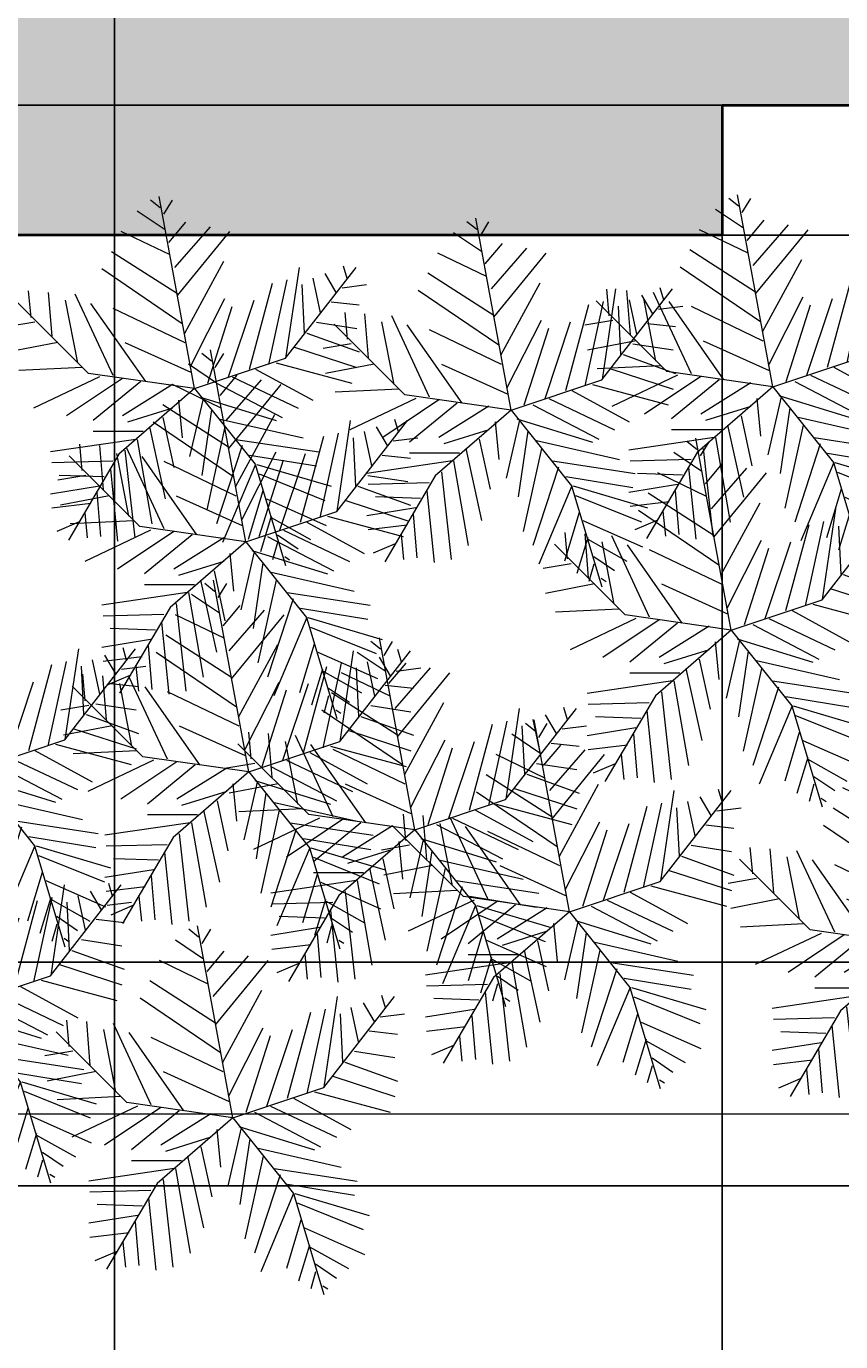
# Model space of a CAD drawing. Units: inches. Extents: x 818 to 1898, y 976 to 2364.
# Tile 39 of 96: x 1622 to 1667, y 1277 to 1350. Entities that reach past the tile are written whole.
import ezdxf

# ---------------------------------------------------------------- set-up
doc = ezdxf.new("R2010")
doc.units = ezdxf.units.IN
doc.header["$LTSCALE"] = 5
doc.header["$MEASUREMENT"] = 0
for name, color, linetype, lineweight in [('A-ANNO-DIMS', 2, 'Continuous', 18), ('A-WALL', 7, 'Continuous', 40), ('L-PLNT-BEDS', 94, 'Continuous', 18)]:
    doc.layers.add(name, color=color, linetype=linetype, lineweight=lineweight)
doc.layers.add('A-WALL-PATT', color=251, linetype='Continuous', lineweight=13, true_color=0x636466)
doc.layers.add('L-PLNT', color=116, linetype='Continuous', lineweight=13, true_color=0x136734)
doc.styles.get("Standard").update_dxf_attribs({"font": 'arial.ttf'})
doc.dimstyles.get("Standard").update_dxf_attribs({"dimtxt": 0.18, "dimasz": 0.18, "dimexe": 0.18, "dimexo": 0.0625, "dimgap": 0.09, "dimtad": 0, "dimtih": 1, "dimtoh": 1, "dimdec": 4, "dimzin": 0, "dimdsep": 46, "dimtxsty": 'Standard', "dimcen": 0.09, "dimadec": 0, "dimazin": 0, "dimtfac": 1, "dimtdec": 4, "dimtofl": 0, "dimtmove": 0, "dimatfit": 3, "dimfxl": 1, "dimtolj": 1, "dimtzin": 0, "dimarcsym": 0})

# ---------------------------------------------------------------- blocks, each defined once
blk = doc.blocks.new('SHRUB-ACCENT')
for p, q in [((10.438, 9.815), (8.475, 20.472)), ((8.533, 19.844), (7.992, 20.278)), ((8.737, 19.496), (9.211, 20.278)), ((8.804, 18.628), (7.247, 19.67)), ((9.008, 17.934), (9.956, 19.062)), ((9.075, 17.239), (6.366, 18.541)), ((9.346, 16.544), (11.31, 18.802)), ((9.482, 14.981), (12.394, 18.541)), ((9.482, 15.068), (5.824, 17.413)), ((9.888, 12.898), (12.055, 16.892)), ((9.753, 13.419), (5.283, 16.458)), ((15.486, 11.498), (19.412, 16.546)), ((15.509, 11.509), (16.254, 16.544)), ((17.677, 16.197), (18.286, 15.155)), ((18.693, 16.631), (18.896, 15.937)), ((13.478, 10.901), (14.764, 15.676)), ((14.561, 11.161), (15.577, 15.85)), ((16.39, 15.589), (16.525, 12.898)), ((16.999, 15.937), (17.406, 14.026)), ((18.625, 15.416), (19.979, 15.589)), ((1.354, 13.766), (1.219, 15.242)), ((2.303, 15.155), (2.506, 12.724)), ((3.251, 14.721), (3.928, 11.248)), ((3.793, 15.068), (5.892, 10.553)), ((10.227, 11.074), (12.123, 14.808)), ((12.326, 10.467), (13.748, 14.721)), ((18.015, 14.634), (19.573, 14.461)), ((4.549, 10.657), (0.623, 14.583)), ((7.721, 10.206), (4.673, 14.547)), ((5.892, 14.287), (9.888, 12.377)), ((11.175, 10.119), (12.529, 14.374)), ((1.558, 13.505), (0, 13.245)), ((17.203, 13.505), (19.437, 13.158)), ((16.661, 12.898), (19.573, 11.856)), ((2.845, 12.377), (0.136, 11.856)), ((6.569, 12.377), (10.227, 10.727)), ((15.983, 12.116), (19.437, 10.988)), ((4.199, 10.988), (0.677, 10.814)), ((10.438, 9.815), (15.486, 11.498)), ((14.968, 11.248), (19.166, 10.119)), ((5.147, 10.467), (1.49, 8.73)), ((6.434, 10.38), (3.319, 8.296)), ((10.438, 9.815), (4.549, 10.657)), ((12.529, 10.467), (16.187, 8.73)), ((13.816, 10.901), (16.999, 9.164)), ((7.45, 10.206), (4.809, 8.035)), ((10.438, 9.815), (6.231, 6.17)), ((9.211, 10.033), (6.434, 8.296)), ((10.438, 9.815), (13.803, 5.609)), ((11.649, 10.119), (15.306, 8.209)), ((9.549, 9.164), (9.753, 7.08)), ((10.904, 9.251), (10.159, 6.039)), ((10.769, 9.338), (14.968, 8.035)), ((9.211, 8.73), (6.705, 7.949)), ((8.669, 8.209), (9.278, 5.431)), ((11.378, 8.643), (10.836, 4.997)), ((11.852, 8.122), (16.457, 7.08)), ((7.585, 7.428), (4.809, 7.428)), ((7.924, 7.688), (8.804, 3.694)), ((12.123, 7.688), (11.107, 3.086)), ((7.179, 6.994), (2.438, 6.299)), ((7.247, 6.994), (8.06, 2.305)), ((13.071, 6.646), (11.649, 2.305)), ((12.733, 6.994), (17.338, 6.299)), ((6.231, 6.17), (3.427, 1.402)), ((6.569, 6.386), (7.111, 1.524)), ((13.478, 6.125), (17.203, 5.517)), ((5.892, 5.778), (2.506, 5.691)), ((5.757, 5.344), (6.163, 1.35)), ((13.816, 5.604), (11.988, 1.263)), ((13.803, 5.609), (15.486, 0)), ((13.884, 5.604), (18.015, 4.389)), ((5.147, 4.389), (2.438, 3.955)), ((5.418, 4.91), (2.912, 4.997)), ((14.019, 5.083), (17.677, 3.607)), ((5.012, 4.041), (5.215, 1.61)), ((14.223, 4.128), (13.41, 1.437)), ((14.426, 3.694), (17.744, 2.218)), ((4.673, 3.434), (2.506, 3.173)), ((3.996, 2.392), (2.777, 1.871)), ((4.334, 2.913), (4.47, 1.524)), ((14.697, 2.739), (14.087, 0.742)), ((14.697, 2.652), (16.864, 1.437)), ((15.035, 1.697), (16.187, 0.916)), ((15.035, 1.263), (14.764, 0.308)), ((15.442, 0.482), (15.712, 0.308))]:
    blk.add_line(p, q)
blk = doc.blocks.new('*D65')
at = {"layer": 'A-ANNO-DIMS', "color": 0, "lineweight": -2, "ltscale": 5, "transparency": 16777216}
for p, q in [((1430.725, 1346.016), (1430.725, 975.663)), ((1714.725, 1346.016), (1714.725, 975.663)), ((1430.905, 975.843), (1572.435, 975.843)), ((1714.545, 975.843), (1573.015, 975.843))]:
    blk.add_line(p, q, dxfattribs=at)
at = {"layer": 'A-ANNO-DIMS', "color": 0, "ltscale": 5, "transparency": 16777216}
for points in [[(1430.905, 975.873), (1430.905, 975.813), (1430.725, 975.843)], [(1714.545, 975.873), (1714.545, 975.813), (1714.725, 975.843)]]:
    blk.add_solid(points, dxfattribs=at)
at = {"layer": 'Defpoints', "color": 0, "ltscale": 5, "transparency": 16777216}
for p in [(1430.725, 1346.078), (1714.725, 1346.078), (1714.725, 975.843)]:
    blk.add_point(p, dxfattribs=at)
at = {"layer": 'A-ANNO-DIMS', "color": 0, "ltscale": 5, "transparency": 16777216, "insert": (1572.725, 975.843), "char_height": 0.18, "attachment_point": 5}
blk.add_mtext('\\A1;284', dxfattribs=at)
blk = doc.blocks.new('*D102')
at = {"layer": 'A-ANNO-DIMS', "color": 0, "lineweight": -2, "ltscale": 5, "transparency": 16777216}
for p, q in [((1565.483, 1071.118), (1565.483, 2363.873)), ((1565.663, 2363.693), (1595.635, 2363.693)), ((1626.395, 2363.693), (1596.423, 2363.693)), ((1626.575, 1071.118), (1626.575, 2363.873))]:
    blk.add_line(p, q, dxfattribs=at)
at = {"layer": 'A-ANNO-DIMS', "color": 0, "ltscale": 5, "transparency": 16777216}
for points in [[(1565.663, 2363.723), (1565.663, 2363.663), (1565.483, 2363.693)], [(1626.395, 2363.723), (1626.395, 2363.663), (1626.575, 2363.693)]]:
    blk.add_solid(points, dxfattribs=at)
at = {"layer": 'Defpoints', "color": 0, "ltscale": 5, "transparency": 16777216}
for p in [(1626.575, 2363.693), (1565.483, 1071.055), (1626.575, 1071.055)]:
    blk.add_point(p, dxfattribs=at)
at = {"layer": 'A-ANNO-DIMS', "color": 0, "ltscale": 5, "transparency": 16777216, "insert": (1596.029, 2363.693), "char_height": 0.18, "attachment_point": 5}
blk.add_mtext('\\A1;61.09', dxfattribs=at)
blk = doc.blocks.new('*D103')
at = {"layer": 'A-ANNO-DIMS', "color": 0, "lineweight": -2, "ltscale": 5, "transparency": 16777216}
for p, q in [((1626.575, 1071.118), (1626.575, 2363.873)), ((1626.755, 2363.693), (1657.699, 2363.693)), ((1689.291, 2363.693), (1658.348, 2363.693)), ((1689.471, 1071.118), (1689.471, 2363.873))]:
    blk.add_line(p, q, dxfattribs=at)
at = {"layer": 'A-ANNO-DIMS', "color": 0, "ltscale": 5, "transparency": 16777216}
for points in [[(1626.755, 2363.723), (1626.755, 2363.663), (1626.575, 2363.693)], [(1689.291, 2363.723), (1689.291, 2363.663), (1689.471, 2363.693)]]:
    blk.add_solid(points, dxfattribs=at)
at = {"layer": 'Defpoints', "color": 0, "ltscale": 5, "transparency": 16777216}
for p in [(1689.471, 2363.693), (1626.575, 1071.055), (1689.471, 1071.055)]:
    blk.add_point(p, dxfattribs=at)
at = {"layer": 'A-ANNO-DIMS', "color": 0, "ltscale": 5, "transparency": 16777216, "insert": (1658.023, 2363.693), "char_height": 0.18, "attachment_point": 5}
blk.add_mtext('\\A1;62.9', dxfattribs=at)
blk = doc.blocks.new('*D113')
at = {"layer": 'A-ANNO-DIMS', "color": 0, "lineweight": -2, "ltscale": 5, "transparency": 16777216}
for p, q in [((1430.788, 1346.078), (1897.916, 1346.078)), ((1897.736, 1345.898), (1897.736, 1316.26)), ((1897.736, 1286.258), (1897.736, 1315.896)), ((1430.788, 1286.078), (1897.916, 1286.078))]:
    blk.add_line(p, q, dxfattribs=at)
at = {"layer": 'A-ANNO-DIMS', "color": 0, "ltscale": 5, "transparency": 16777216}
for points in [[(1897.706, 1345.898), (1897.766, 1345.898), (1897.736, 1346.078)], [(1897.706, 1286.258), (1897.766, 1286.258), (1897.736, 1286.078)]]:
    blk.add_solid(points, dxfattribs=at)
at = {"layer": 'Defpoints', "color": 0, "ltscale": 5, "transparency": 16777216}
for p in [(1430.725, 1346.078), (1897.736, 1346.078), (1430.725, 1286.078)]:
    blk.add_point(p, dxfattribs=at)
at = {"layer": 'A-ANNO-DIMS', "color": 0, "ltscale": 5, "transparency": 16777216, "insert": (1897.736, 1316.078), "char_height": 0.18, "attachment_point": 5}
blk.add_mtext('\\A1;60', dxfattribs=at)
blk = doc.blocks.new('*D115')
at = {"layer": 'A-ANNO-DIMS', "color": 0, "lineweight": -2, "ltscale": 5, "transparency": 16777216}
for p, q in [((1766.29, 1377.656), (818.026, 1377.656)), ((818.206, 1377.476), (818.206, 1338.262)), ((818.206, 1298.684), (818.206, 1337.898)), ((1766.29, 1298.504), (818.026, 1298.504))]:
    blk.add_line(p, q, dxfattribs=at)
at = {"layer": 'A-ANNO-DIMS', "color": 0, "ltscale": 5, "transparency": 16777216}
for points in [[(818.176, 1377.476), (818.236, 1377.476), (818.206, 1377.656)], [(818.176, 1298.684), (818.236, 1298.684), (818.206, 1298.504)]]:
    blk.add_solid(points, dxfattribs=at)
at = {"layer": 'Defpoints', "color": 0, "ltscale": 5, "transparency": 16777216}
for p in [(818.206, 1377.656), (1766.352, 1377.656), (1766.352, 1298.504)]:
    blk.add_point(p, dxfattribs=at)
at = {"layer": 'A-ANNO-DIMS', "color": 0, "ltscale": 5, "transparency": 16777216, "insert": (818.206, 1338.08), "char_height": 0.18, "attachment_point": 5}
blk.add_mtext('\\A1;79.15', dxfattribs=at)
blk = doc.blocks.new('*D180')
at = {"layer": 'A-ANNO-DIMS', "color": 0, "lineweight": -2, "ltscale": 5, "transparency": 16777216}
for p, q in [((1599.725, 1639.516), (1599.725, 975.663)), ((1669.725, 1639.516), (1669.725, 975.663)), ((1599.905, 975.843), (1634.507, 975.843)), ((1669.545, 975.843), (1634.943, 975.843))]:
    blk.add_line(p, q, dxfattribs=at)
at = {"layer": 'A-ANNO-DIMS', "color": 0, "ltscale": 5, "transparency": 16777216}
for points in [[(1599.905, 975.873), (1599.905, 975.813), (1599.725, 975.843)], [(1669.545, 975.873), (1669.545, 975.813), (1669.725, 975.843)]]:
    blk.add_solid(points, dxfattribs=at)
at = {"layer": 'Defpoints', "color": 0, "ltscale": 5, "transparency": 16777216}
for p in [(1599.725, 1639.578), (1669.725, 1639.578), (1669.725, 975.843)]:
    blk.add_point(p, dxfattribs=at)
at = {"layer": 'A-ANNO-DIMS', "color": 0, "ltscale": 5, "transparency": 16777216, "insert": (1634.725, 975.843), "char_height": 0.18, "attachment_point": 5}
blk.add_mtext('\\A1;70', dxfattribs=at)
blk = doc.blocks.new('*D192')
at = {"layer": 'A-ANNO-DIMS', "color": 0, "lineweight": -2, "ltscale": 5, "transparency": 16777216}
for p, q in [((1555.13, 1338.803), (1555.13, 975.663)), ((1660.314, 1338.803), (1660.314, 975.663)), ((1555.31, 975.843), (1607.267, 975.843)), ((1660.134, 975.843), (1608.177, 975.843))]:
    blk.add_line(p, q, dxfattribs=at)
at = {"layer": 'A-ANNO-DIMS', "color": 0, "ltscale": 5, "transparency": 16777216}
for points in [[(1555.31, 975.873), (1555.31, 975.813), (1555.13, 975.843)], [(1660.134, 975.873), (1660.134, 975.813), (1660.314, 975.843)]]:
    blk.add_solid(points, dxfattribs=at)
at = {"layer": 'Defpoints', "color": 0, "ltscale": 5, "transparency": 16777216}
for p in [(1555.13, 1338.865), (1660.314, 1338.865), (1660.314, 975.843)]:
    blk.add_point(p, dxfattribs=at)
at = {"layer": 'A-ANNO-DIMS', "color": 0, "ltscale": 5, "transparency": 16777216, "insert": (1607.722, 975.843), "char_height": 0.18, "attachment_point": 5}
blk.add_mtext('\\A1;105.18', dxfattribs=at)
blk = doc.blocks.new('*D193')
at = {"layer": 'A-ANNO-DIMS', "color": 0, "lineweight": -2, "ltscale": 5, "transparency": 16777216}
for p, q in [((1660.377, 1346.078), (1897.916, 1346.078)), ((1897.736, 1345.898), (1897.736, 1342.654)), ((1897.736, 1339.045), (1897.736, 1342.29)), ((1660.377, 1338.865), (1897.916, 1338.865))]:
    blk.add_line(p, q, dxfattribs=at)
at = {"layer": 'A-ANNO-DIMS', "color": 0, "ltscale": 5, "transparency": 16777216}
for points in [[(1897.706, 1345.898), (1897.766, 1345.898), (1897.736, 1346.078)], [(1897.706, 1339.045), (1897.766, 1339.045), (1897.736, 1338.865)]]:
    blk.add_solid(points, dxfattribs=at)
at = {"layer": 'Defpoints', "color": 0, "ltscale": 5, "transparency": 16777216}
for p in [(1660.314, 1346.078), (1897.736, 1346.078), (1660.314, 1338.865)]:
    blk.add_point(p, dxfattribs=at)
at = {"layer": 'A-ANNO-DIMS', "color": 0, "ltscale": 5, "transparency": 16777216, "insert": (1897.736, 1342.472), "char_height": 0.18, "attachment_point": 5}
blk.add_mtext('\\A1;7.213', dxfattribs=at)
blk = doc.blocks.new('*D198')
at = {"layer": 'A-ANNO-DIMS', "color": 0, "lineweight": -2, "ltscale": 5, "transparency": 16777216}
for p, q in [((1741.841, 1545.016), (1741.841, 975.663)), ((1430.725, 1346.016), (1430.725, 975.663)), ((1430.905, 975.843), (1585.907, 975.843)), ((1741.661, 975.843), (1586.659, 975.843))]:
    blk.add_line(p, q, dxfattribs=at)
at = {"layer": 'A-ANNO-DIMS', "color": 0, "ltscale": 5, "transparency": 16777216}
for points in [[(1430.905, 975.873), (1430.905, 975.813), (1430.725, 975.843)], [(1741.661, 975.873), (1741.661, 975.813), (1741.841, 975.843)]]:
    blk.add_solid(points, dxfattribs=at)
at = {"layer": 'Defpoints', "color": 0, "ltscale": 5, "transparency": 16777216}
for p in [(1741.841, 1545.078), (1430.725, 1346.078), (1741.841, 975.843)]:
    blk.add_point(p, dxfattribs=at)
at = {"layer": 'A-ANNO-DIMS', "color": 0, "ltscale": 5, "transparency": 16777216, "insert": (1586.283, 975.843), "char_height": 0.18, "attachment_point": 5}
blk.add_mtext('\\A1;311.1', dxfattribs=at)
blk = doc.blocks.new('*D199')
at = {"layer": 'A-ANNO-DIMS', "color": 0, "lineweight": -2, "ltscale": 5, "transparency": 16777216}
for p, q in [((1559.788, 1687.078), (1897.916, 1687.078)), ((1897.736, 1686.898), (1897.736, 1513.154)), ((1897.736, 1339.045), (1897.736, 1512.79)), ((1660.377, 1338.865), (1897.916, 1338.865))]:
    blk.add_line(p, q, dxfattribs=at)
at = {"layer": 'A-ANNO-DIMS', "color": 0, "ltscale": 5, "transparency": 16777216}
for points in [[(1897.706, 1686.898), (1897.766, 1686.898), (1897.736, 1687.078)], [(1897.706, 1339.045), (1897.766, 1339.045), (1897.736, 1338.865)]]:
    blk.add_solid(points, dxfattribs=at)
at = {"layer": 'Defpoints', "color": 0, "ltscale": 5, "transparency": 16777216}
for p in [(1559.725, 1687.078), (1897.736, 1687.078), (1660.314, 1338.865)]:
    blk.add_point(p, dxfattribs=at)
at = {"layer": 'A-ANNO-DIMS', "color": 0, "ltscale": 5, "transparency": 16777216, "insert": (1897.736, 1512.972), "char_height": 0.18, "attachment_point": 5}
blk.add_mtext('\\A1;348.2', dxfattribs=at)
blk = doc.blocks.new('*D214')
at = {"layer": 'A-ANNO-DIMS', "color": 0, "lineweight": -2, "ltscale": 5, "transparency": 16777216}
for p, q in [((1511.725, 1687.016), (1511.725, 975.663)), ((1714.725, 1687.016), (1714.725, 975.663)), ((1511.905, 975.843), (1612.935, 975.843)), ((1714.545, 975.843), (1613.516, 975.843))]:
    blk.add_line(p, q, dxfattribs=at)
at = {"layer": 'A-ANNO-DIMS', "color": 0, "ltscale": 5, "transparency": 16777216}
for points in [[(1511.905, 975.873), (1511.905, 975.813), (1511.725, 975.843)], [(1714.545, 975.873), (1714.545, 975.813), (1714.725, 975.843)]]:
    blk.add_solid(points, dxfattribs=at)
at = {"layer": 'Defpoints', "color": 0, "ltscale": 5, "transparency": 16777216}
for p in [(1511.725, 1687.078), (1714.725, 1687.078), (1714.725, 975.843)]:
    blk.add_point(p, dxfattribs=at)
at = {"layer": 'A-ANNO-DIMS', "color": 0, "ltscale": 5, "transparency": 16777216, "insert": (1613.225, 975.843), "char_height": 0.18, "attachment_point": 5}
blk.add_mtext('\\A1;203', dxfattribs=at)

msp = doc.modelspace()

# ---------------------------------------------------------------- hatches: boundary and pattern name
at = {"layer": 'A-WALL-PATT', "ltscale": 5}
h = msp.add_hatch(color=256, dxfattribs=at)
h.dxf.hatch_style = 1
h.paths.add_polyline_path([(1714.7251, 1521.0782), (1705.7252, 1521.0782), (1705.7252, 1467.0782), (1654.7252, 1467.0782), (1654.7252, 1463.0782), (1705.7252, 1463.0782), (1705.7252, 1355.0782), (1622.7252, 1355.0782), (1622.7252, 1379.0782), (1622.7252, 1386.6857), (1616.7252, 1386.6857), (1616.7252, 1355.0782), (1490.9163, 1355.0782), (1490.9163, 1346.0782), (1544.7605, 1346.0782), (1544.6132, 1346.8783), (1544.6729, 1346.84), (1544.6299, 1346.7874), (1544.7605, 1346.0782), (1555.1299, 1346.0782), (1555.1299, 1341.5528), (1556.1599, 1340.8639), (1556.5281, 1338.8654), (1660.3141, 1338.8654), (1660.3141, 1346.0782), (1705.7252, 1346.0782), (1705.7252, 1345.0768), (1705.8704, 1344.58), (1705.7252, 1344.3933), (1705.7252, 1334.9904), (1705.8704, 1334.4936), (1705.7252, 1334.3068), (1705.7252, 1316.2253), (1707.3573, 1316.7694), (1707.3847, 1316.8046), (1707.3807, 1316.7771), (1705.7252, 1316.2253), (1705.7252, 1314.1392), (1705.7252, 1312.0957), (1705.8703, 1312.0739), (1705.7252, 1311.8873), (1705.7252, 1310.7121), (1706.5603, 1307.9282), (1707.8887, 1307.1831), (1714.7251, 1307.1831), (1714.7251, 1346.0782)])

# ---------------------------------------------------------------- linework, layer by layer
at = {"layer": 'A-WALL'}
msp.add_line((1660.3141, 1346.0782), (1705.7252, 1346.0782), dxfattribs=at)
at = {"layer": 'A-WALL', "ltscale": 5}
msp.add_lwpolyline([(1660.3141, 1346.0782), (1660.3141, 1338.8654), (1555.1299, 1338.8654), (1555.1299, 1346.0782)], dxfattribs=at)
at = {"layer": 'L-PLNT-BEDS', "ltscale": 5}
for points in [[(1430.7251, 1286.0782), (1701.3688, 1286.0782, 0.4142136), (1713.3688, 1298.0782), (1713.3688, 1307.1831)], [(1430.7251, 1290.0782), (1701.3688, 1290.0782, 0.4142136), (1709.3688, 1298.0782), (1709.3688, 1307.1831)]]:
    msp.add_lwpolyline(points, format="xyb", dxfattribs=at)

# ---------------------------------------------------------------- block references
at = {"layer": 'L-PLNT'}
for p in [(1620.5869, 1320.5352), (1652.6968, 1320.6323), (1638.1568, 1319.3368), (1623.4315, 1312.0264), (1650.3815, 1307.122), (1608.3357, 1299.349), (1623.5991, 1299.2462), (1632.8099, 1296.0338), (1641.3982, 1291.4834), (1660.6615, 1289.6327), (1607.5406, 1286.2497), (1622.7082, 1280.0457)]:
    msp.add_blockref('SHRUB-ACCENT', p, dxfattribs=at)

# ---------------------------------------------------------------- dimensions: what is measured, and where the dimension line sits
at = {"layer": 'A-ANNO-DIMS', "ltscale": 5}
for base, p1, p2, override, picture, middle in [((1626.5748, 2363.6929), (1565.4835, 1071.0552), (1626.5748, 1071.0552), {"dimdec": 2, "dimlfac": 1, "dimrnd": 0, "dimzin": 0, "dimdsep": 46, "dimlunit": 2}, '*D102', (1596.0291, 2363.6929)), ((1689.4714, 2363.6929), (1626.5748, 1071.0552), (1689.4714, 1071.0552), {"dimdec": 1, "dimlfac": 1, "dimrnd": 0, "dimzin": 0, "dimdsep": 46, "dimlunit": 2}, '*D103', (1658.0231, 2363.6929)), ((1714.7251, 975.8433), (1511.7251, 1687.0782), (1714.7251, 1687.0782), {"dimdec": 0, "dimlfac": 1, "dimrnd": 0, "dimzin": 0, "dimdsep": 46, "dimlunit": 2}, '*D214', (1613.2251, 975.8433)), ((1669.7251, 975.8433), (1599.7251, 1639.5782), (1669.7251, 1639.5782), {"dimdec": 0, "dimlfac": 1, "dimrnd": 0, "dimzin": 0, "dimdsep": 46, "dimlunit": 2}, '*D180', (1634.7251, 975.8433)), ((1741.8409, 975.8433), (1430.7251, 1346.0782), (1741.8409, 1545.0782), {"dimdec": 1, "dimlfac": 1, "dimrnd": 0, "dimzin": 0, "dimdsep": 46, "dimlunit": 2}, '*D198', (1586.283, 975.8433)), ((1714.7251, 975.8433), (1430.7251, 1346.0782), (1714.7251, 1346.0782), {"dimdec": 0, "dimlfac": 1, "dimrnd": 0, "dimzin": 0, "dimdsep": 46, "dimlunit": 2}, '*D65', (1572.7251, 975.8433)), ((1660.3141, 975.8433), (1555.1299, 1338.8654), (1660.3141, 1338.8654), {"dimdec": 2, "dimlfac": 1, "dimrnd": 0, "dimzin": 0, "dimdsep": 46, "dimlunit": 2}, '*D192', (1607.722, 975.8433))]:
    dim = msp.add_linear_dim(base=base, p1=p1, p2=p2, dimstyle='Standard', override=override, dxfattribs=at)
    dim.commit()
    dim.dimension.update_dxf_attribs({"geometry": picture, "text_midpoint": middle})
for base, p1, p2, override, picture, middle in [((1897.736, 1687.0782), (1660.3141, 1338.8654), (1559.7251, 1687.0782), {"dimdec": 1, "dimlfac": 1, "dimrnd": 0, "dimzin": 0, "dimdsep": 46, "dimlunit": 2}, '*D199', (1897.736, 1512.9718)), ((818.2059, 1377.6564), (1766.3524, 1298.5041), (1766.3524, 1377.6564), {"dimdec": 2, "dimlfac": 1, "dimrnd": 0, "dimzin": 0, "dimdsep": 46, "dimlunit": 2}, '*D115', (818.2059, 1338.0803)), ((1897.736, 1346.0782), (1430.7251, 1286.0782), (1430.7251, 1346.0782), {"dimdec": 0, "dimlfac": 1, "dimrnd": 0, "dimzin": 0, "dimdsep": 46, "dimlunit": 2}, '*D113', (1897.736, 1316.0782)), ((1897.736, 1346.0782), (1660.3141, 1338.8654), (1660.3141, 1346.0782), {"dimdec": 3, "dimlfac": 1, "dimrnd": 0, "dimzin": 0, "dimdsep": 46, "dimlunit": 2}, '*D193', (1897.736, 1342.4718))]:
    dim = msp.add_linear_dim(base=base, p1=p1, p2=p2, angle=90, dimstyle='Standard', override=override, dxfattribs=at)
    dim.commit()
    dim.dimension.update_dxf_attribs({"geometry": picture, "text_midpoint": middle})

doc.saveas('drawing.dxf')
